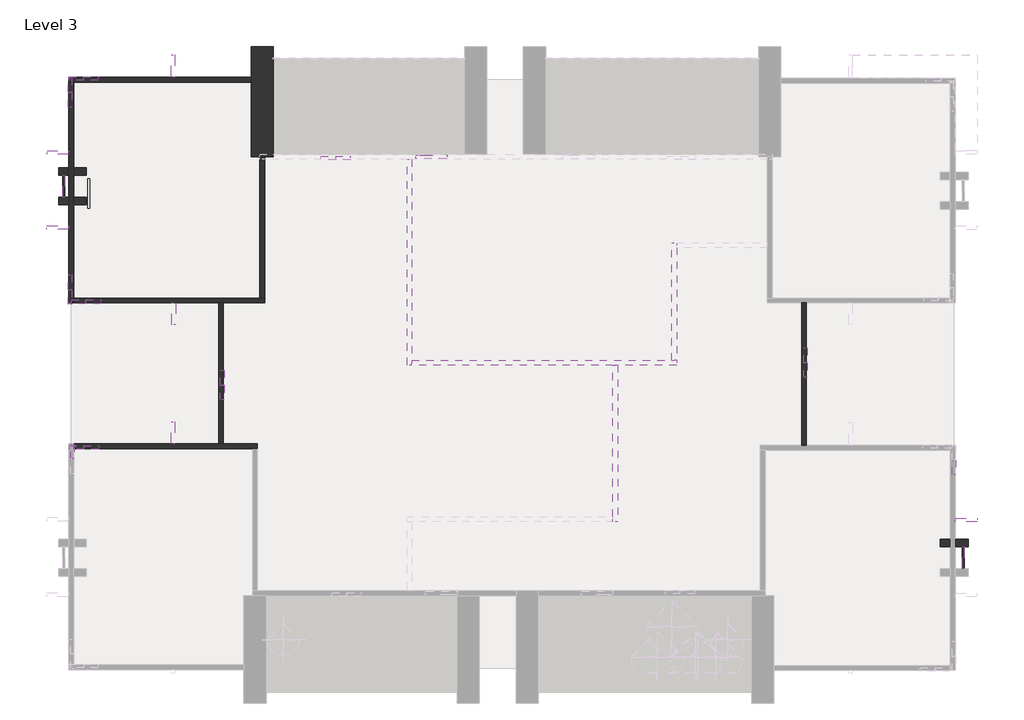
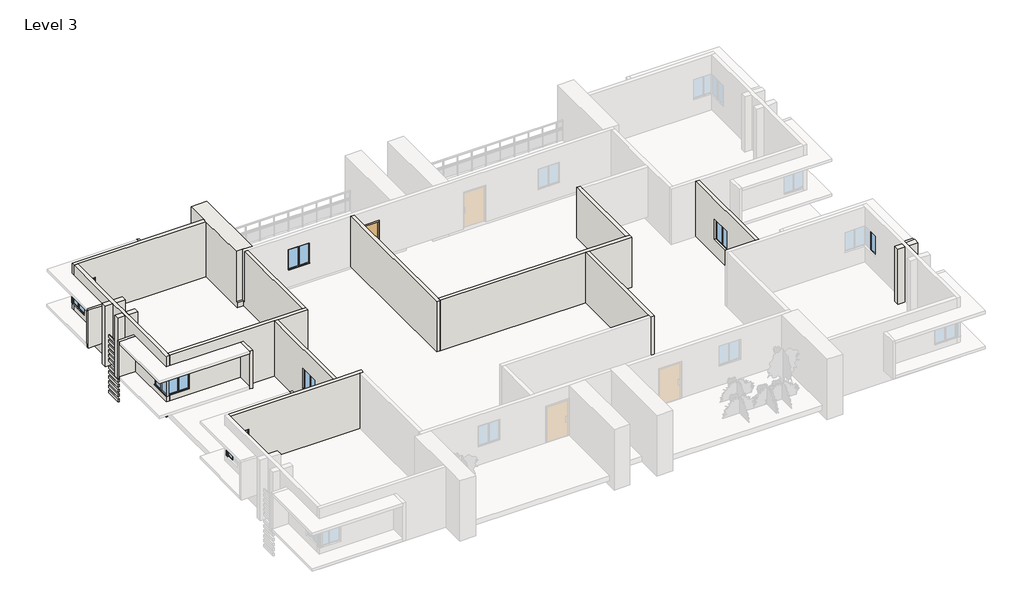
# One storey, part 2 of 4: 49 walls, 18 windows, 1 door.
"""IFC4 building model written with IfcOpenShell, lengths in millimetres."""

from ifc_helpers import new_model, si_unit, frame, origin, place, context, project, spatial, polyline, outline, extrude, faceted_brep, transform, mapped, element, save
from components import door_15d3c954, window_20ff4747

model = new_model("IFC4")

# Units and contexts
model_context = context("Model", 3, world=origin())
ifc_project = project(units=[si_unit("LENGTHUNIT", "METRE", prefix="MILLI")], contexts=[model_context])

# Site, building, storey
site = spatial("IfcSite", under=ifc_project)
building = spatial("IfcBuilding", under=site)
storey = spatial("IfcBuildingStorey", under=building, Name="Level 3", Elevation=6096.0)

# Door
placement = place(None, origin())
door_shape = door_15d3c954(model_context)
element("IfcDoor", 1, ObjectType="Door-Passage-Single-Flush-Dbl_Acting : 48\" x 96\"", at=placement, inside=storey, context=model_context, shape_type="MappedRepresentation", body=[
    mapped(door_shape, transform((153.0520665, 12804.5205944, 7315.2), x_axis=(1.0, 0.0, 0.0), y_axis=(0.0, 1.0, 0.0), z_axis=(0.0, 0.0, 1.0))),
])

# Walls
element("IfcWall", 2, ObjectType="Generic - 1'", at=placement, inside=storey, context=model_context, shape_type="SweptSolid", body=[
    extrude(outline(polyline([(-14151.7972154, 12048.8705944), (-14667.8479335, 12048.8705944), (-14667.8479335, 12353.6705944), (-14151.7972154, 12353.6705944), (-14151.7972154, 12048.8705944)])), frame((0.0, 0.0, 6705.6), z_axis=(0.0, 0.0, 1.0), x_axis=(1.0, 0.0, 0.0)), (0.0, 0.0, 1.0), 3657.6),
])
element("IfcWall", 3, ObjectType="Generic - 1'", at=placement, inside=storey, context=model_context, shape_type="SweptSolid", body=[
    extrude(outline(polyline([(-15302.1394029, 12353.6705944), (-14871.0479335, 12353.6705944), (-14871.0479335, 12048.8705944), (-15302.1394029, 12048.8705944), (-15302.1394029, 12353.6705944)])), frame((0.0, 0.0, 6705.6), z_axis=(0.0, 0.0, 1.0), x_axis=(1.0, 0.0, 0.0)), (0.0, 0.0, 1.0), 3657.6),
])
element("IfcWall", 4, ObjectType="Generic - 1'", at=placement, inside=storey, context=model_context, shape_type="SweptSolid", body=[
    extrude(outline(polyline([(-14151.7972154, 10829.6705944), (-14667.8479335, 10829.6705944), (-14667.8479335, 11134.4705944), (-14151.7972154, 11134.4705944), (-14151.7972154, 10829.6705944)])), frame((0.0, 0.0, 6705.6), z_axis=(0.0, 0.0, 1.0), x_axis=(1.0, 0.0, 0.0)), (0.0, 0.0, 1.0), 3657.6),
])
element("IfcWall", 5, ObjectType="Generic - 1'", at=placement, inside=storey, context=model_context, shape_type="SweptSolid", body=[
    extrude(outline(polyline([(-15302.1394029, 11134.4705944), (-14871.0479335, 11134.4705944), (-14871.0479335, 10829.6705944), (-15302.1394029, 10829.6705944), (-15302.1394029, 11134.4705944)])), frame((0.0, 0.0, 6705.6), z_axis=(0.0, 0.0, 1.0), x_axis=(1.0, 0.0, 0.0)), (0.0, 0.0, 1.0), 3657.6),
])
element("IfcWall", 6, ObjectType="Generic - 1'", at=placement, inside=storey, context=model_context, shape_type="SweptSolid", body=[
    extrude(outline(polyline([(22386.1027846, -3343.5294056), (21857.3520665, -3343.5294056), (21857.3520665, -3038.7294056), (22386.1027846, -3038.7294056), (22386.1027846, -3343.5294056)])), frame((0.0, 0.0, 6705.6), z_axis=(0.0, 0.0, 1.0), x_axis=(1.0, 0.0, 0.0)), (0.0, 0.0, 1.0), 3657.6),
])
element("IfcWall", 7, ObjectType="Generic - 1'", at=placement, inside=storey, context=model_context, shape_type="SweptSolid", body=[
    extrude(outline(polyline([(21235.7605971, -3038.7294056), (21654.1520665, -3038.7294056), (21654.1520665, -3343.5294056), (21235.7605971, -3343.5294056), (21235.7605971, -3038.7294056)])), frame((0.0, 0.0, 6705.6), z_axis=(0.0, 0.0, 1.0), x_axis=(1.0, 0.0, 0.0)), (0.0, 0.0, 1.0), 3657.6),
])
element("IfcWall", 8, ObjectType="Generic - 3'", at=placement, inside=storey, context=model_context, shape_type="Brep", body=[
    faceted_brep([(-6400.1479335, 12810.8705944, 6705.6), (-6400.1479335, 17382.8705944, 6705.6), (-6400.1479335, 17382.8705944, 10363.2), (-6400.1479335, 12912.4705944, 10363.2), (-6400.1479335, 12912.4705944, 7315.2), (-6400.1479335, 12810.8705944, 7315.2), (-7314.5479335, 12810.8705944, 6705.6), (-7314.5479335, 12810.8705944, 7315.2), (-7314.5479335, 12912.4705944, 7315.2), (-7314.5479335, 12912.4705944, 10363.2), (-7314.5479335, 15904.9548886, 10363.2), (-7314.5479335, 16108.1548886, 10363.2), (-7314.5479335, 17382.8705944, 10363.2), (-7314.5479335, 17382.8705944, 6705.6), (-7314.5479335, 16108.1548886, 6705.6), (-7314.5479335, 15904.9548886, 6705.6), (-6755.7479335, 12810.8705944, 6705.6), (-6958.9479335, 12810.8705944, 6705.6), (-6958.9479335, 12912.4705944, 10363.2), (-6755.7479335, 12810.8705944, 7315.2), (-6958.9479335, 12810.8705944, 7315.2), (-6958.9479335, 12912.4705944, 7315.2)], [[[0, 1, 2, 3, 4, 5]], [[6, 7, 8, 9, 10, 11, 12, 13, 14, 15]], [[1, 0, 16, 17, 6, 15, 14, 13]], [[2, 1, 13, 12]], [[3, 2, 12, 11, 10, 9, 18]], [[0, 5, 19, 20, 7, 6, 17, 16]], [[4, 21, 8, 7, 20, 19, 5]], [[4, 3, 18, 9, 8, 21]]]),
])
element("IfcWall", 9, ObjectType="Generic - 5\"", at=placement, inside=storey, context=model_context, shape_type="SweptSolid", body=[
    extrude(outline(polyline([(-15124.6936682, 11134.4705944), (-15124.6936682, 12048.8705944), (-15048.4936682, 12048.8705944), (-15048.4936682, 11134.4705944), (-15124.6936682, 11134.4705944)])), frame((0.0, 0.0, 5054.6), z_axis=(0.0, 0.0, 1.0), x_axis=(1.0, 0.0, 0.0)), (0.0, 0.0, 1.0), 152.8735856),
])
element("IfcWall", 10, ObjectType="Generic - 5\"", at=placement, inside=storey, context=model_context, shape_type="SweptSolid", body=[
    extrude(outline(polyline([(-15124.6936682, 11134.4705944), (-15124.6936682, 12048.8705944), (-15048.4936682, 12048.8705944), (-15048.4936682, 11134.4705944), (-15124.6936682, 11134.4705944)])), frame((0.0, 0.0, 5359.4), z_axis=(0.0, 0.0, 1.0), x_axis=(1.0, 0.0, 0.0)), (0.0, 0.0, 1.0), 152.8735856),
])
element("IfcWall", 11, ObjectType="Generic - 5\"", at=placement, inside=storey, context=model_context, shape_type="SweptSolid", body=[
    extrude(outline(polyline([(-15124.6936682, 11134.4705944), (-15124.6936682, 12048.8705944), (-15048.4936682, 12048.8705944), (-15048.4936682, 11134.4705944), (-15124.6936682, 11134.4705944)])), frame((0.0, 0.0, 5638.8), z_axis=(0.0, 0.0, 1.0), x_axis=(1.0, 0.0, 0.0)), (0.0, 0.0, 1.0), 152.8735856),
])
element("IfcWall", 12, ObjectType="Generic - 5\"", at=placement, inside=storey, context=model_context, shape_type="SweptSolid", body=[
    extrude(outline(polyline([(-15124.6936682, 11134.4705944), (-15124.6936682, 12048.8705944), (-15048.4936682, 12048.8705944), (-15048.4936682, 11134.4705944), (-15124.6936682, 11134.4705944)])), frame((0.0, 0.0, 5943.6), z_axis=(0.0, 0.0, 1.0), x_axis=(1.0, 0.0, 0.0)), (0.0, 0.0, 1.0), 152.8735856),
])
element("IfcWall", 13, ObjectType="Generic - 5\"", at=placement, inside=storey, context=model_context, shape_type="SweptSolid", body=[
    extrude(outline(polyline([(-15124.6936682, 11134.4705944), (-15124.6936682, 12048.8705944), (-15048.4936682, 12048.8705944), (-15048.4936682, 11134.4705944), (-15124.6936682, 11134.4705944)])), frame((0.0, 0.0, 6248.4), z_axis=(0.0, 0.0, 1.0), x_axis=(1.0, 0.0, 0.0)), (0.0, 0.0, 1.0), 152.8735856),
])
element("IfcWall", 14, ObjectType="Generic - 5\"", at=placement, inside=storey, context=model_context, shape_type="SweptSolid", body=[
    extrude(outline(polyline([(-15124.6936682, 11134.4705944), (-15124.6936682, 12048.8705944), (-15048.4936682, 12048.8705944), (-15048.4936682, 11134.4705944), (-15124.6936682, 11134.4705944)])), frame((0.0, 0.0, 6553.2), z_axis=(0.0, 0.0, 1.0), x_axis=(1.0, 0.0, 0.0)), (0.0, 0.0, 1.0), 152.8735856),
])
element("IfcWall", 15, ObjectType="Generic - 5\"", at=placement, inside=storey, context=model_context, shape_type="SweptSolid", body=[
    extrude(outline(polyline([(22145.9857703, -4257.9294056), (22145.9857703, -3343.5294056), (22222.1857703, -3343.5294056), (22222.1857703, -4257.9294056), (22145.9857703, -4257.9294056)])), frame((0.0, 0.0, 5054.6), z_axis=(0.0, 0.0, 1.0), x_axis=(1.0, 0.0, 0.0)), (0.0, 0.0, 1.0), 152.8735856),
])
element("IfcWall", 16, ObjectType="Generic - 5\"", at=placement, inside=storey, context=model_context, shape_type="SweptSolid", body=[
    extrude(outline(polyline([(22145.9857703, -4257.9294056), (22145.9857703, -3343.5294056), (22222.1857703, -3343.5294056), (22222.1857703, -4257.9294056), (22145.9857703, -4257.9294056)])), frame((0.0, 0.0, 5359.4), z_axis=(0.0, 0.0, 1.0), x_axis=(1.0, 0.0, 0.0)), (0.0, 0.0, 1.0), 152.8735856),
])
element("IfcWall", 17, ObjectType="Generic - 5\"", at=placement, inside=storey, context=model_context, shape_type="SweptSolid", body=[
    extrude(outline(polyline([(22145.9857703, -4257.9294056), (22145.9857703, -3343.5294056), (22222.1857703, -3343.5294056), (22222.1857703, -4257.9294056), (22145.9857703, -4257.9294056)])), frame((0.0, 0.0, 5638.8), z_axis=(0.0, 0.0, 1.0), x_axis=(1.0, 0.0, 0.0)), (0.0, 0.0, 1.0), 152.8735856),
])
element("IfcWall", 18, ObjectType="Generic - 5\"", at=placement, inside=storey, context=model_context, shape_type="SweptSolid", body=[
    extrude(outline(polyline([(22145.9857703, -4257.9294056), (22145.9857703, -3343.5294056), (22222.1857703, -3343.5294056), (22222.1857703, -4257.9294056), (22145.9857703, -4257.9294056)])), frame((0.0, 0.0, 5943.6), z_axis=(0.0, 0.0, 1.0), x_axis=(1.0, 0.0, 0.0)), (0.0, 0.0, 1.0), 152.8735856),
])
element("IfcWall", 19, ObjectType="Generic - 5\"", at=placement, inside=storey, context=model_context, shape_type="SweptSolid", body=[
    extrude(outline(polyline([(22145.9857703, -4257.9294056), (22145.9857703, -3343.5294056), (22222.1857703, -3343.5294056), (22222.1857703, -4257.9294056), (22145.9857703, -4257.9294056)])), frame((0.0, 0.0, 6248.4), z_axis=(0.0, 0.0, 1.0), x_axis=(1.0, 0.0, 0.0)), (0.0, 0.0, 1.0), 152.8735856),
])
element("IfcWall", 20, ObjectType="Generic - 5\"", at=placement, inside=storey, context=model_context, shape_type="SweptSolid", body=[
    extrude(outline(polyline([(22145.9857703, -4257.9294056), (22145.9857703, -3343.5294056), (22222.1857703, -3343.5294056), (22222.1857703, -4257.9294056), (22145.9857703, -4257.9294056)])), frame((0.0, 0.0, 6553.2), z_axis=(0.0, 0.0, 1.0), x_axis=(1.0, 0.0, 0.0)), (0.0, 0.0, 1.0), 152.8735856),
])
element("IfcWall", 21, ObjectType="Generic - 5\"", at=placement, inside=storey, context=model_context, shape_type="SweptSolid", body=[
    extrude(outline(polyline([(-15124.6936682, 11134.4705944), (-15124.6936682, 12048.8705944), (-15048.4936682, 12048.8705944), (-15048.4936682, 11134.4705944), (-15124.6936682, 11134.4705944)])), frame((0.0, 0.0, 6959.6), z_axis=(0.0, 0.0, 1.0), x_axis=(1.0, 0.0, 0.0)), (0.0, 0.0, 1.0), 152.8735856),
])
element("IfcWall", 22, ObjectType="Generic - 5\"", at=placement, inside=storey, context=model_context, shape_type="SweptSolid", body=[
    extrude(outline(polyline([(-14084.4224108, 10677.2705944), (-14084.4224108, 11896.4705944), (-14008.2224108, 11896.4705944), (-14008.2224108, 10677.2705944), (-14084.4224108, 10677.2705944)])), frame((0.0, 0.0, 6959.6), z_axis=(0.0, 0.0, 1.0), x_axis=(1.0, 0.0, 0.0)), (0.0, 0.0, 1.0), 178.1810075),
])
element("IfcWall", 23, ObjectType="Generic - 5\"", at=placement, inside=storey, context=model_context, shape_type="SweptSolid", body=[
    extrude(outline(polyline([(-15124.6936682, 11134.4705944), (-15124.6936682, 12048.8705944), (-15048.4936682, 12048.8705944), (-15048.4936682, 11134.4705944), (-15124.6936682, 11134.4705944)])), frame((0.0, 0.0, 7239.0), z_axis=(0.0, 0.0, 1.0), x_axis=(1.0, 0.0, 0.0)), (0.0, 0.0, 1.0), 152.8735856),
])
element("IfcWall", 24, ObjectType="Generic - 5\"", at=placement, inside=storey, context=model_context, shape_type="SweptSolid", body=[
    extrude(outline(polyline([(-15124.6936682, 11134.4705944), (-15124.6936682, 12048.8705944), (-15048.4936682, 12048.8705944), (-15048.4936682, 11134.4705944), (-15124.6936682, 11134.4705944)])), frame((0.0, 0.0, 7518.4), z_axis=(0.0, 0.0, 1.0), x_axis=(1.0, 0.0, 0.0)), (0.0, 0.0, 1.0), 152.8735856),
])
element("IfcWall", 25, ObjectType="Generic - 5\"", at=placement, inside=storey, context=model_context, shape_type="SweptSolid", body=[
    extrude(outline(polyline([(-15124.6936682, 11134.4705944), (-15124.6936682, 12048.8705944), (-15048.4936682, 12048.8705944), (-15048.4936682, 11134.4705944), (-15124.6936682, 11134.4705944)])), frame((0.0, 0.0, 7823.2), z_axis=(0.0, 0.0, 1.0), x_axis=(1.0, 0.0, 0.0)), (0.0, 0.0, 1.0), 152.8735856),
])
element("IfcWall", 26, ObjectType="Generic - 5\"", at=placement, inside=storey, context=model_context, shape_type="SweptSolid", body=[
    extrude(outline(polyline([(-15124.6936682, 11134.4705944), (-15124.6936682, 12048.8705944), (-15048.4936682, 12048.8705944), (-15048.4936682, 11134.4705944), (-15124.6936682, 11134.4705944)])), frame((0.0, 0.0, 8128.0), z_axis=(0.0, 0.0, 1.0), x_axis=(1.0, 0.0, 0.0)), (0.0, 0.0, 1.0), 152.8735856),
])
element("IfcWall", 27, ObjectType="Generic - 5\"", at=placement, inside=storey, context=model_context, shape_type="SweptSolid", body=[
    extrude(outline(polyline([(-15124.6936682, 11134.4705944), (-15124.6936682, 12048.8705944), (-15048.4936682, 12048.8705944), (-15048.4936682, 11134.4705944), (-15124.6936682, 11134.4705944)])), frame((0.0, 0.0, 8407.4), z_axis=(0.0, 0.0, 1.0), x_axis=(1.0, 0.0, 0.0)), (0.0, 0.0, 1.0), 152.8735856),
])
element("IfcWall", 28, ObjectType="Generic - 5\"", at=placement, inside=storey, context=model_context, shape_type="SweptSolid", body=[
    extrude(outline(polyline([(22145.9857703, -4257.9294056), (22145.9857703, -3343.5294056), (22222.1857703, -3343.5294056), (22222.1857703, -4257.9294056), (22145.9857703, -4257.9294056)])), frame((0.0, 0.0, 6959.6), z_axis=(0.0, 0.0, 1.0), x_axis=(1.0, 0.0, 0.0)), (0.0, 0.0, 1.0), 152.8735856),
])
element("IfcWall", 29, ObjectType="Generic - 5\"", at=placement, inside=storey, context=model_context, shape_type="SweptSolid", body=[
    extrude(outline(polyline([(22145.9857703, -4257.9294056), (22145.9857703, -3343.5294056), (22222.1857703, -3343.5294056), (22222.1857703, -4257.9294056), (22145.9857703, -4257.9294056)])), frame((0.0, 0.0, 7239.0), z_axis=(0.0, 0.0, 1.0), x_axis=(1.0, 0.0, 0.0)), (0.0, 0.0, 1.0), 152.8735856),
])
element("IfcWall", 30, ObjectType="Generic - 5\"", at=placement, inside=storey, context=model_context, shape_type="SweptSolid", body=[
    extrude(outline(polyline([(22145.9857703, -4257.9294056), (22145.9857703, -3343.5294056), (22222.1857703, -3343.5294056), (22222.1857703, -4257.9294056), (22145.9857703, -4257.9294056)])), frame((0.0, 0.0, 7518.4), z_axis=(0.0, 0.0, 1.0), x_axis=(1.0, 0.0, 0.0)), (0.0, 0.0, 1.0), 152.8735856),
])
element("IfcWall", 31, ObjectType="Generic - 5\"", at=placement, inside=storey, context=model_context, shape_type="SweptSolid", body=[
    extrude(outline(polyline([(22145.9857703, -4257.9294056), (22145.9857703, -3343.5294056), (22222.1857703, -3343.5294056), (22222.1857703, -4257.9294056), (22145.9857703, -4257.9294056)])), frame((0.0, 0.0, 7823.2), z_axis=(0.0, 0.0, 1.0), x_axis=(1.0, 0.0, 0.0)), (0.0, 0.0, 1.0), 152.8735856),
])
element("IfcWall", 32, ObjectType="Generic - 5\"", at=placement, inside=storey, context=model_context, shape_type="SweptSolid", body=[
    extrude(outline(polyline([(22145.9857703, -4257.9294056), (22145.9857703, -3343.5294056), (22222.1857703, -3343.5294056), (22222.1857703, -4257.9294056), (22145.9857703, -4257.9294056)])), frame((0.0, 0.0, 8128.0), z_axis=(0.0, 0.0, 1.0), x_axis=(1.0, 0.0, 0.0)), (0.0, 0.0, 1.0), 152.8735856),
])
element("IfcWall", 33, ObjectType="Generic - 5\"", at=placement, inside=storey, context=model_context, shape_type="SweptSolid", body=[
    extrude(outline(polyline([(22145.9857703, -4257.9294056), (22145.9857703, -3343.5294056), (22222.1857703, -3343.5294056), (22222.1857703, -4257.9294056), (22145.9857703, -4257.9294056)])), frame((0.0, 0.0, 8407.4), z_axis=(0.0, 0.0, 1.0), x_axis=(1.0, 0.0, 0.0)), (0.0, 0.0, 1.0), 152.8735856),
])
element("IfcWall", 34, ObjectType="Generic - 6\"", at=placement, inside=storey, context=model_context, shape_type="SweptSolid", body=[
    extrude(outline(polyline([(-10480.7034654, 17035.2548886), (-10480.7034654, 16120.8548886), (-10633.1034654, 16120.8548886), (-10633.1034654, 17035.2548886), (-10480.7034654, 17035.2548886)])), frame((0.0, 0.0, 7467.6), z_axis=(0.0, 0.0, 1.0), x_axis=(1.0, 0.0, 0.0)), (0.0, 0.0, 1.0), 2286.0),
])
element("IfcWall", 35, ObjectType="Generic - 6\"", at=placement, inside=storey, context=model_context, shape_type="SweptSolid", body=[
    extrude(outline(polyline([(-15775.8097154, 13072.8548886), (-14883.7479335, 13072.8548886), (-14883.7479335, 12920.4548886), (-15775.8097154, 12920.4548886), (-15775.8097154, 13072.8548886)])), frame((0.0, 0.0, 7467.6), z_axis=(0.0, 0.0, 1.0), x_axis=(1.0, 0.0, 0.0)), (0.0, 0.0, 1.0), 2286.0),
])
element("IfcWall", 36, ObjectType="Generic - 6\"", at=placement, inside=storey, context=model_context, shape_type="SweptSolid", body=[
    extrude(outline(polyline([(-10603.8479335, 5846.5548886), (-10603.8479335, 6760.9548886), (-10451.4479335, 6760.9548886), (-10451.4479335, 5846.5548886), (-10603.8479335, 5846.5548886)])), frame((0.0, 0.0, 7467.6), z_axis=(0.0, 0.0, 1.0), x_axis=(1.0, 0.0, 0.0)), (0.0, 0.0, 1.0), 2286.0),
])
element("IfcWall", 37, ObjectType="Generic - 6\"", at=placement, inside=storey, context=model_context, shape_type="SweptSolid", body=[
    extrude(outline(polyline([(-15798.1479335, 9961.3548886), (-14883.7479335, 9961.3548886), (-14883.7479335, 9808.9548886), (-15798.1479335, 9808.9548886), (-15798.1479335, 9961.3548886)])), frame((0.0, 0.0, 7467.6), z_axis=(0.0, 0.0, 1.0), x_axis=(1.0, 0.0, 0.0)), (0.0, 0.0, 1.0), 2286.0),
])
element("IfcWall", 38, ObjectType="Generic - 6\"", at=placement, inside=storey, context=model_context, shape_type="SweptSolid", body=[
    extrude(outline(polyline([(-10480.7034654, 1834.0395301), (-10480.7034654, 919.6395301), (-10633.1034654, 919.6395301), (-10633.1034654, 1834.0395301), (-10480.7034654, 1834.0395301)])), frame((0.0, 0.0, 7467.6), z_axis=(0.0, 0.0, 1.0), x_axis=(1.0, 0.0, 0.0)), (0.0, 0.0, 1.0), 2286.0),
])
element("IfcWall", 39, ObjectType="Generic - 6\"", at=placement, inside=storey, context=model_context, shape_type="SweptSolid", body=[
    extrude(outline(polyline([(22771.7520665, -2309.5899195), (21857.3520665, -2309.5899195), (21857.3520665, -2157.1899195), (22771.7520665, -2157.1899195), (22771.7520665, -2309.5899195)])), frame((0.0, 0.0, 7467.6), z_axis=(0.0, 0.0, 1.0), x_axis=(1.0, 0.0, 0.0)), (0.0, 0.0, 1.0), 2286.0),
])
element("IfcWall", 40, ObjectType="Generic - 8\"", at=placement, inside=storey, context=model_context, shape_type="Brep", body=[
    faceted_brep([(-862.9479335, 12709.2705944, 7315.2), (-862.9479335, 4174.8705944, 7315.2), (-862.9479335, 4174.8705944, 10363.2), (-862.9479335, 12709.2705944, 10363.2), (-659.7479335, 12709.2705944, 7315.2), (-659.7479335, 12709.2705944, 10363.2), (-659.7479335, 4378.0705944, 10363.2), (-659.7479335, 4174.8705944, 10363.2), (-659.7479335, 4174.8705944, 7315.2), (-659.7479335, 4378.0705944, 7315.2)], [[[0, 1, 2, 3]], [[4, 5, 6, 7, 8, 9]], [[1, 0, 4, 9, 8]], [[3, 2, 7, 6, 5]], [[0, 3, 5, 4]], [[2, 1, 8, 7]]]),
])
element("IfcWall", 41, ObjectType="Generic - 8\"", at=placement, inside=storey, context=model_context, shape_type="Brep", body=[
    faceted_brep([(-659.7479335, 4174.8705944, 7315.2), (7671.4520665, 4174.8705944, 7315.2), (7874.6520665, 4174.8705944, 7315.2), (10313.0520665, 4174.8705944, 7315.2), (10313.0520665, 4174.8705944, 10363.2), (7874.6520665, 4174.8705944, 10363.2), (7671.4520665, 4174.8705944, 10363.2), (-659.7479335, 4174.8705944, 10363.2), (-659.7479335, 4378.0705944, 7315.2), (-659.7479335, 4378.0705944, 10363.2), (10109.8520665, 4378.0705944, 10363.2), (10313.0520665, 4378.0705944, 10363.2), (10313.0520665, 4378.0705944, 7315.2), (10109.8520665, 4378.0705944, 7315.2)], [[[0, 1, 2, 3, 4, 5, 6, 7]], [[8, 9, 10, 11, 12, 13]], [[3, 2, 1, 0, 8, 13, 12]], [[7, 6, 5, 4, 11, 10, 9]], [[0, 7, 9, 8]], [[4, 3, 12, 11]]]),
])
element("IfcWall", 42, ObjectType="Generic - 8\"", at=placement, inside=storey, context=model_context, shape_type="Brep", body=[
    faceted_brep([(10313.0520665, 4378.0705944, 7315.2), (10313.0520665, 9051.6705944, 7315.2), (10313.0520665, 9254.8705944, 7315.2), (10313.0520665, 9254.8705944, 10363.2), (10313.0520665, 9051.6705944, 10363.2), (10313.0520665, 4378.0705944, 10363.2), (10109.8520665, 4378.0705944, 7315.2), (10109.8520665, 4378.0705944, 10363.2), (10109.8520665, 9254.8705944, 10363.2), (10109.8520665, 9254.8705944, 7315.2)], [[[0, 1, 2, 3, 4, 5]], [[6, 7, 8, 9]], [[2, 1, 0, 6, 9]], [[5, 4, 3, 8, 7]], [[0, 5, 7, 6]], [[3, 2, 9, 8]]]),
])
element("IfcWall", 43, ObjectType="Generic - 8\"", at=placement, inside=storey, context=model_context, shape_type="Brep", body=[
    faceted_brep([(7671.4520665, 4174.8705944, 7315.2), (7671.4520665, -2102.9604699, 7315.2), (7671.4520665, -2306.1604699, 7315.2), (7671.4520665, -2306.1604699, 10363.2), (7671.4520665, -2102.9604699, 10363.2), (7671.4520665, 4174.8705944, 10363.2), (7874.6520665, 4174.8705944, 7315.2), (7874.6520665, 4174.8705944, 10363.2), (7874.6520665, -2306.1604699, 10363.2), (7874.6520665, -2306.1604699, 7315.2)], [[[0, 1, 2, 3, 4, 5]], [[6, 7, 8, 9]], [[2, 1, 0, 6, 9]], [[5, 4, 3, 8, 7]], [[0, 5, 7, 6]], [[3, 2, 9, 8]]]),
])
element("IfcWall", 44, ObjectType="Generic - 8\" gray", at=placement, inside=storey, context=model_context, shape_type="Brep", body=[
    faceted_brep([(-14871.0479335, 15904.9548886, 6705.6), (-14667.8479335, 15904.9548886, 6705.6), (-7314.5479335, 15904.9548886, 6705.6), (-7314.5479335, 15904.9548886, 10363.2), (-14667.8479335, 15904.9548886, 10363.2), (-14871.0479335, 15904.9548886, 10363.2), (-14871.0479335, 15904.9548886, 9197.0804451), (-14667.8479335, 15904.9548886, 9197.0804451), (-13661.292575, 15904.9548886, 9197.0804451), (-13661.292575, 15904.9548886, 7977.8804451), (-14667.8479335, 15904.9548886, 7977.8804451), (-14871.0479335, 15904.9548886, 7977.8804451), (-7314.5479335, 16108.1548886, 6705.6), (-14871.0479335, 16108.1548886, 6705.6), (-14871.0479335, 16108.1548886, 7977.8804451), (-13661.292575, 16108.1548886, 7977.8804451), (-13661.292575, 16108.1548886, 9197.0804451), (-14871.0479335, 16108.1548886, 9197.0804451), (-14871.0479335, 16108.1548886, 10363.2), (-7314.5479335, 16108.1548886, 10363.2)], [[[0, 1, 2, 3, 4, 5, 6, 7, 8, 9, 10, 11]], [[12, 13, 14, 15, 16, 17, 18, 19]], [[2, 1, 0, 13, 12]], [[5, 4, 3, 19, 18]], [[5, 18, 17, 6]], [[13, 0, 11, 14]], [[3, 2, 12, 19]], [[9, 15, 14, 11, 10]], [[6, 17, 16, 8, 7]], [[8, 16, 15, 9]]]),
])
element("IfcWall", 45, ObjectType="Generic - 8\" gray", at=placement, inside=storey, context=model_context, shape_type="Brep", body=[
    faceted_brep([(-14667.8479335, 6760.9548886, 6705.6), (-14667.8479335, 6964.1548886, 6705.6), (-14667.8479335, 10829.6705944, 6705.6), (-14667.8479335, 11134.4705944, 6705.6), (-14667.8479335, 12048.8705944, 6705.6), (-14667.8479335, 12353.6705944, 6705.6), (-14667.8479335, 15904.9548886, 6705.6), (-14667.8479335, 15904.9548886, 7977.8804451), (-14667.8479335, 14871.0236266, 7977.8804451), (-14667.8479335, 14871.0236266, 9197.0804451), (-14667.8479335, 15904.9548886, 9197.0804451), (-14667.8479335, 15904.9548886, 10363.2), (-14667.8479335, 12353.6705944, 10363.2), (-14667.8479335, 12048.8705944, 10363.2), (-14667.8479335, 11134.4705944, 10363.2), (-14667.8479335, 10829.6705944, 10363.2), (-14667.8479335, 6964.1548886, 10363.2), (-14667.8479335, 6760.9548886, 10363.2), (-14667.8479335, 6760.9548886, 9197.0804451), (-14667.8479335, 6964.1548886, 9197.0804451), (-14667.8479335, 7918.4820466, 9197.0804451), (-14667.8479335, 7918.4820466, 7977.8804451), (-14667.8479335, 6964.1548886, 7977.8804451), (-14667.8479335, 6760.9548886, 7977.8804451), (-14871.0479335, 15904.9548886, 6705.6), (-14871.0479335, 12353.6705944, 6705.6), (-14871.0479335, 12048.8705944, 6705.6), (-14871.0479335, 11134.4705944, 6705.6), (-14871.0479335, 10829.6705944, 6705.6), (-14871.0479335, 6760.9548886, 6705.6), (-14871.0479335, 6760.9548886, 7977.8804451), (-14871.0479335, 7918.4820466, 7977.8804451), (-14871.0479335, 7918.4820466, 9197.0804451), (-14871.0479335, 6760.9548886, 9197.0804451), (-14871.0479335, 6760.9548886, 10363.2), (-14871.0479335, 10829.6705944, 10363.2), (-14871.0479335, 11134.4705944, 10363.2), (-14871.0479335, 12048.8705944, 10363.2), (-14871.0479335, 12353.6705944, 10363.2), (-14871.0479335, 15904.9548886, 10363.2), (-14871.0479335, 15904.9548886, 9197.0804451), (-14871.0479335, 14871.0236266, 9197.0804451), (-14871.0479335, 14871.0236266, 7977.8804451), (-14871.0479335, 15904.9548886, 7977.8804451)], [[[0, 1, 2, 3, 4, 5, 6, 7, 8, 9, 10, 11, 12, 13, 14, 15, 16, 17, 18, 19, 20, 21, 22, 23]], [[24, 25, 26, 27, 28, 29, 30, 31, 32, 33, 34, 35, 36, 37, 38, 39, 40, 41, 42, 43]], [[6, 5, 4, 3, 2, 1, 0, 29, 28, 27, 26, 25, 24]], [[17, 16, 15, 14, 13, 12, 11, 39, 38, 37, 36, 35, 34]], [[17, 34, 33, 18]], [[29, 0, 23, 30]], [[6, 24, 43, 7]], [[39, 11, 10, 40]], [[30, 23, 22, 21, 31]], [[18, 33, 32, 20, 19]], [[20, 32, 31, 21]], [[7, 43, 42, 8]], [[9, 8, 42, 41]], [[9, 41, 40, 10]]]),
])
element("IfcWall", 46, ObjectType="Generic - 8\" gray", at=placement, inside=storey, context=model_context, shape_type="Brep", body=[
    faceted_brep([(-6755.7479335, 6964.1548886, 6705.6), (-6958.9479335, 6964.1548886, 6705.6), (-14667.8479335, 6964.1548886, 6705.6), (-14667.8479335, 6964.1548886, 7977.8804451), (-13556.3228261, 6964.1548886, 7977.8804451), (-13556.3228261, 6964.1548886, 9197.0804451), (-14667.8479335, 6964.1548886, 9197.0804451), (-14667.8479335, 6964.1548886, 10363.2), (-6958.9479335, 6964.1548886, 10363.2), (-6755.7479335, 6964.1548886, 10363.2), (-14667.8479335, 6760.9548886, 6705.6), (-8673.4479335, 6760.9548886, 6705.6), (-8470.2479335, 6760.9548886, 6705.6), (-6755.7479335, 6760.9548886, 6705.6), (-6755.7479335, 6760.9548886, 10363.2), (-8470.2479335, 6760.9548886, 10363.2), (-8673.4479335, 6760.9548886, 10363.2), (-14667.8479335, 6760.9548886, 10363.2), (-14667.8479335, 6760.9548886, 9197.0804451), (-13556.3228261, 6760.9548886, 9197.0804451), (-13556.3228261, 6760.9548886, 7977.8804451), (-14667.8479335, 6760.9548886, 7977.8804451)], [[[0, 1, 2, 3, 4, 5, 6, 7, 8, 9]], [[10, 11, 12, 13, 14, 15, 16, 17, 18, 19, 20, 21]], [[2, 1, 0, 13, 12, 11, 10]], [[9, 8, 7, 17, 16, 15, 14]], [[2, 10, 21, 3]], [[17, 7, 6, 18]], [[0, 9, 14, 13]], [[3, 21, 20, 4]], [[5, 4, 20, 19]], [[5, 19, 18, 6]]]),
])
element("IfcWall", 47, ObjectType="Generic - 8\" gray", at=placement, inside=storey, context=model_context, shape_type="Brep", body=[
    faceted_brep([(-7060.5479335, 919.6395301, 6705.6), (-8470.2479335, 919.6395301, 6705.6), (-8673.4479335, 919.6395301, 6705.6), (-14680.5479335, 919.6395301, 6705.6), (-14680.5479335, 919.6395301, 7977.8804451), (-13641.9760869, 919.6395301, 7977.8804451), (-13641.9760869, 919.6395301, 9197.0804451), (-14680.5479335, 919.6395301, 9197.0804451), (-14680.5479335, 919.6395301, 10363.2), (-8673.4479335, 919.6395301, 10363.2), (-8470.2479335, 919.6395301, 10363.2), (-7060.5479335, 919.6395301, 10363.2), (-14680.5479335, 716.4395301, 6705.6), (-7263.7479335, 716.4395301, 6705.6), (-7060.5479335, 716.4395301, 6705.6), (-7060.5479335, 716.4395301, 10363.2), (-7263.7479335, 716.4395301, 10363.2), (-14680.5479335, 716.4395301, 10363.2), (-14680.5479335, 716.4395301, 9197.0804451), (-13641.9760869, 716.4395301, 9197.0804451), (-13641.9760869, 716.4395301, 7977.8804451), (-14680.5479335, 716.4395301, 7977.8804451), (-14680.5479335, 908.9135189, 7977.8804451), (-14680.5479335, 908.9135189, 9197.0804451)], [[[0, 1, 2, 3, 4, 5, 6, 7, 8, 9, 10, 11]], [[12, 13, 14, 15, 16, 17, 18, 19, 20, 21]], [[3, 2, 1, 0, 14, 13, 12]], [[11, 10, 9, 8, 17, 16, 15]], [[3, 12, 21, 22, 4]], [[17, 8, 7, 23, 18]], [[0, 11, 15, 14]], [[4, 22, 21, 20, 5]], [[6, 5, 20, 19]], [[6, 19, 18, 23, 7]]]),
])
element("IfcWall", 48, ObjectType="Generic - 8\" gray", at=placement, inside=storey, context=model_context, shape_type="SweptSolid", body=[
    extrude(outline(polyline([(6760.9548886, 6705.6), (919.6395301, 6705.6), (919.6395301, 10363.2), (6760.9548886, 10363.2), (6760.9548886, 6705.6)]), holes=[polyline([(2742.9076732, 7977.8804451), (3962.1076732, 7977.8804451), (3962.1076732, 9197.0804451), (2742.9076732, 9197.0804451), (2742.9076732, 7977.8804451)])]), frame((-8673.4479335, 0.0, 0.0), z_axis=(1.0, 0.0, 0.0), x_axis=(0.0, 1.0, 0.0)), (0.0, 0.0, 1.0), 203.2),
])
element("IfcWall", 49, ObjectType="Generic - 8\" gray", at=placement, inside=storey, context=model_context, shape_type="SweptSolid", body=[
    extrude(outline(polyline([(6760.9548886, 6705.6), (868.1548886, 6705.6), (868.1548886, 10363.2), (6760.9548886, 10363.2), (6760.9548886, 6705.6)]), holes=[polyline([(3676.3636585, 7977.8804451), (4895.5636585, 7977.8804451), (4895.5636585, 9197.0804451), (3676.3636585, 9197.0804451), (3676.3636585, 7977.8804451)])]), frame((15481.9520665, 0.0, 0.0), z_axis=(1.0, 0.0, 0.0), x_axis=(0.0, 1.0, 0.0)), (0.0, 0.0, 1.0), 203.2),
])
element("IfcWall", 50, ObjectType="Generic - 8\" gray", at=placement, inside=storey, context=model_context, shape_type="SweptSolid", body=[
    extrude(outline(polyline([(6964.1548886, 6705.6), (6964.1548886, 10363.2), (12709.2705944, 10363.2), (12709.2705944, 7315.2), (12810.8705944, 7315.2), (12810.8705944, 6705.6), (6964.1548886, 6705.6)])), frame((-6958.9479335, 0.0, 0.0), z_axis=(1.0, 0.0, 0.0), x_axis=(0.0, 1.0, 0.0)), (0.0, 0.0, 1.0), 203.2),
])

# Windows
window_shape = window_20ff4747(model_context)
element("IfcWindow", 51, ObjectType="Instance - Fixed : 24\" x 48\"", at=placement, inside=storey, context=model_context, shape_type="MappedRepresentation", body=[
    mapped(window_shape, transform((21755.7520665, -93.135515, 7063.4804451), x_axis=(0.0, -1.0, 0.0), y_axis=(1.0, 0.0, 0.0), z_axis=(0.0, 0.0, 1.0))),
])
element("IfcWindow", 52, ObjectType="Instance - Fixed : 24\" x 48\"", at=placement, inside=storey, context=model_context, shape_type="MappedRepresentation", body=[
    mapped(window_shape, transform((-14782.1479335, 566.0135189, 7063.4804451), x_axis=(0.0, -1.0, 0.0), y_axis=(1.0, 0.0, 0.0), z_axis=(0.0, 0.0, 1.0))),
])
element("IfcWindow", 53, ObjectType="Instance - Fixed : 24\" x 48\"", at=placement, inside=storey, context=model_context, shape_type="MappedRepresentation", body=[
    mapped(window_shape, transform((-14594.4760869, 818.0395301, 7063.4804451), x_axis=(-1.0, 0.0, 0.0), y_axis=(0.0, -1.0, 0.0), z_axis=(0.0, 0.0, 1.0))),
])
element("IfcWindow", 54, ObjectType="Instance - Fixed : 24\" x 48\"", at=placement, inside=storey, context=model_context, shape_type="MappedRepresentation", body=[
    mapped(window_shape, transform((-13984.8760869, 818.0395301, 7063.4804451), x_axis=(-1.0, 0.0, 0.0), y_axis=(0.0, -1.0, 0.0), z_axis=(0.0, 0.0, 1.0))),
])
element("IfcWindow", 55, ObjectType="Instance - Fixed : 24\" x 48\"", at=placement, inside=storey, context=model_context, shape_type="MappedRepresentation", body=[
    mapped(window_shape, transform((-14508.8228261, 6862.5548886, 7063.4804451), x_axis=(-1.0, 0.0, 0.0), y_axis=(0.0, -1.0, 0.0), z_axis=(0.0, 0.0, 1.0))),
])
element("IfcWindow", 56, ObjectType="Instance - Fixed : 24\" x 48\"", at=placement, inside=storey, context=model_context, shape_type="MappedRepresentation", body=[
    mapped(window_shape, transform((-13899.2228261, 6862.5548886, 7063.4804451), x_axis=(-1.0, 0.0, 0.0), y_axis=(0.0, -1.0, 0.0), z_axis=(0.0, 0.0, 1.0))),
])
element("IfcWindow", 57, ObjectType="Instance - Fixed : 24\" x 48\"", at=placement, inside=storey, context=model_context, shape_type="MappedRepresentation", body=[
    mapped(window_shape, transform((-14769.4479335, 7651.7820466, 7063.4804451), x_axis=(0.0, 1.0, 0.0), y_axis=(-1.0, 0.0, 0.0), z_axis=(0.0, 0.0, 1.0))),
])
element("IfcWindow", 58, ObjectType="Instance - Fixed : 24\" x 48\"", at=placement, inside=storey, context=model_context, shape_type="MappedRepresentation", body=[
    mapped(window_shape, transform((-14769.4479335, 7042.1820466, 7063.4804451), x_axis=(0.0, 1.0, 0.0), y_axis=(-1.0, 0.0, 0.0), z_axis=(0.0, 0.0, 1.0))),
])
element("IfcWindow", 59, ObjectType="Instance - Fixed : 24\" x 48\"", at=placement, inside=storey, context=model_context, shape_type="MappedRepresentation", body=[
    mapped(window_shape, transform((-14769.4479335, 15823.5236266, 7063.4804451), x_axis=(0.0, 1.0, 0.0), y_axis=(-1.0, 0.0, 0.0), z_axis=(0.0, 0.0, 1.0))),
])
element("IfcWindow", 60, ObjectType="Instance - Fixed : 24\" x 48\"", at=placement, inside=storey, context=model_context, shape_type="MappedRepresentation", body=[
    mapped(window_shape, transform((-14769.4479335, 15213.9236266, 7063.4804451), x_axis=(0.0, 1.0, 0.0), y_axis=(-1.0, 0.0, 0.0), z_axis=(0.0, 0.0, 1.0))),
])
element("IfcWindow", 61, ObjectType="Instance - Fixed : 24\" x 48\"", at=placement, inside=storey, context=model_context, shape_type="MappedRepresentation", body=[
    mapped(window_shape, transform((-13927.992575, 16006.5548886, 7063.4804451), x_axis=(1.0, 0.0, 0.0), y_axis=(0.0, 1.0, 0.0), z_axis=(0.0, 0.0, 1.0))),
])
element("IfcWindow", 62, ObjectType="Instance - Fixed : 24\" x 48\"", at=placement, inside=storey, context=model_context, shape_type="MappedRepresentation", body=[
    mapped(window_shape, transform((-14537.592575, 16006.5548886, 7063.4804451), x_axis=(1.0, 0.0, 0.0), y_axis=(0.0, 1.0, 0.0), z_axis=(0.0, 0.0, 1.0))),
])
element("IfcWindow", 63, ObjectType="Instance - Fixed : 24\" x 48\"", at=placement, inside=storey, context=model_context, shape_type="MappedRepresentation", body=[
    mapped(window_shape, transform((-4165.821881, 12810.8705944, 7446.2298362), x_axis=(-1.0, 0.0, 0.0), y_axis=(0.0, -1.0, 0.0), z_axis=(0.0, 0.0, 1.0))),
])
element("IfcWindow", 64, ObjectType="Instance - Fixed : 24\" x 48\"", at=placement, inside=storey, context=model_context, shape_type="MappedRepresentation", body=[
    mapped(window_shape, transform((-3556.221881, 12810.8705944, 7446.2298362), x_axis=(-1.0, 0.0, 0.0), y_axis=(0.0, -1.0, 0.0), z_axis=(0.0, 0.0, 1.0))),
])
element("IfcWindow", 65, ObjectType="Instance - Fixed : 24\" x 48\"", at=placement, inside=storey, context=model_context, shape_type="MappedRepresentation", body=[
    mapped(window_shape, transform((-8571.8479335, 3009.6076732, 7063.4804451), x_axis=(0.0, -1.0, 0.0), y_axis=(1.0, 0.0, 0.0), z_axis=(0.0, 0.0, 1.0))),
])
element("IfcWindow", 66, ObjectType="Instance - Fixed : 24\" x 48\"", at=placement, inside=storey, context=model_context, shape_type="MappedRepresentation", body=[
    mapped(window_shape, transform((-8571.8479335, 3619.2076732, 7063.4804451), x_axis=(0.0, -1.0, 0.0), y_axis=(1.0, 0.0, 0.0), z_axis=(0.0, 0.0, 1.0))),
])
element("IfcWindow", 67, ObjectType="Instance - Fixed : 24\" x 48\"", at=placement, inside=storey, context=model_context, shape_type="MappedRepresentation", body=[
    mapped(window_shape, transform((15583.5520665, 3943.0636585, 7063.4804451), x_axis=(0.0, -1.0, 0.0), y_axis=(1.0, 0.0, 0.0), z_axis=(0.0, 0.0, 1.0))),
])
element("IfcWindow", 68, ObjectType="Instance - Fixed : 24\" x 48\"", at=placement, inside=storey, context=model_context, shape_type="MappedRepresentation", body=[
    mapped(window_shape, transform((15583.5520665, 4552.6636585, 7063.4804451), x_axis=(0.0, -1.0, 0.0), y_axis=(1.0, 0.0, 0.0), z_axis=(0.0, 0.0, 1.0))),
])

save(model, "model.ifc")

# Revit data of these elements
# Type "Door-Passage-Single-Flush-Dbl_Acting : 48\" x 96\""
#   Type Mark = "12"
#   Assembly Code = "B2030200"
#   Analytic Construction = "Wooden"
#   Thickness = 0' - 1 3/4"
#   Thermal Resistance (R) = 2.5876 (h·ft²·°F)/BTU
#   Swing Angle [instance default] = 45.00°
#   Strike Height = 3' - 4"
#   Rough Width [instance default] = 4' - 4"
#   Rough Height [instance default] = 7' - 4"
#   MF Opening Height [instance default] = 0' - 4"
#   MF Opening Width [instance default] = 0' - 4"
#   Inset Calculate [instance default] = 0' - 4"
#   Masonry Inset [instance default] = 0' - 1"
#   Height = 7' - 0"
#   Width = 4' - 0"
#   Heat Transfer Coefficient (U) = 0.3865 BTU/(h·ft²·°F)
#   Masonry Frame Depth = 0' - 5 3/4"
#   Masonry Frame [instance default] = yes
#   Function = 1
#   Dry Wall Frame [instance default] = no
#   Panel Material = Wood - Birch
#   Frame Material = Metal - Paint Finish - Grey
#   Door Handle Material = Aluminum
#   Visual Light Transmittance = 0
#   Solar Heat Gain Coefficient = 0
#   Wall Closure = (empty or 0)
# Type "Generic - 1'"
#   Assembly Code = "B2010"
#   Layers, outside or top first: 1' - 0" "Metal - Painted - Grey" (function 1)
# Type "Generic - 3'"
#   Assembly Code = "B2010"
#   Layers, outside or top first: 3' - 0" "Metal - Painted - Grey" (function 1)
# Type "Generic - 5\""
#   Assembly Code = "B2010"
#   Layers, outside or top first: 0' - 3" "Oak Flooring" (function 1)
# Type "Generic - 6\""
#   Assembly Code = "B2010"
#   Layers, outside or top first: 0' - 6" "Metal - Painted - Grey" (function 1)
# Type "Generic - 8\""
#   Assembly Code = "B2010"
#   Layers, outside or top first: 0' - 8" no material (function 1)
# Type "Generic - 8\" gray"
#   Assembly Code = "B2010"
#   Layers, outside or top first: 0' - 8" "Parking Stripe" (function 1)
# Type "Instance - Fixed : 24\" x 48\""
#   Type Mark = "11"
#   Construction Type Id = "GSP4R"
#   Assembly Code = "B2020100"
#   Analytic Construction = "1/8 in Pilkington single glazing"
#   Visual Light Transmittance = 0.9
#   Thermal Resistance (R) = 0.8466 (h·ft²·°F)/BTU
#   Solar Heat Gain Coefficient = 0.86
#   Heat Transfer Coefficient (U) = 1.1812 BTU/(h·ft²·°F)
#   Height [instance default] = 4' - 0"
#   Default Sill Height = 3' - 0"
#   Width [instance default] = 2' - 0"
#   Window Inset = 0' - 2"
#   Define Thermal Properties by = 1
#   Glass Pane Material = Glass
#   Sash Material = Iron, Ductile
#   Wall Closure = (empty or 0)
# Element 1 (IfcDoor, "Door-Passage-Single-Flush-Dbl_Acting : 48\" x 96\"")
#   Swing Angle = 45.00°
#   Rough Width = 4' - 4"
#   Rough Height = 7' - 4"
#   Masonry Inset = 0' - 1"
#   MF Opening Width = 0' - 4"
#   MF Opening Height = 0' - 4"
#   Inset Calculate = 0' - 4"
#   Masonry Frame = yes
#   Dry Wall Frame = no
#   Phase Created = New Construction
#   Materials on its faces: "Aluminum", "Metal - Paint Finish - Grey", "Wood - Birch"
# Elements 2, 3, 4, 5, 6, 7 (IfcWall, "Generic - 1'")
#   built-in parameter 1001111 = 2' - 0"
#   Top Offset = 0' - 0"
#   Base Offset = 2' - 0"
#   Unconnected Height = 12' - 0"
#   wall height = 12' - 0"
#   Phase Created = New Construction
#   Base Constraint = Level 3
#   Materials on its faces: "Metal - Painted - Grey"
# Element 8 (IfcWall, "Generic - 3'")
#   built-in parameter 1001111 = 2' - 0"
#   Top Offset = 0' - 0"
#   Base Offset = 2' - 0"
#   Unconnected Height = 12' - 0"
#   wall height = 12' - 0"
#   Phase Created = New Construction
#   Base Constraint = Level 3
#   Materials on its faces: "Metal - Painted - Grey", "EIFS, Exterior Insulation"
# Elements 9, 15 (IfcWall, "Generic - 5\"")
#   built-in parameter 1001111 = -3' - 5"
#   Top Offset = -12' - 10.98135"
#   Base Offset = -3' - 5"
#   wall height = 0' - 6.01865"
#   Phase Created = New Construction
#   Base Constraint = Level 3
#   Top Constraint = Level 4
#   Materials on its faces: "Oak Flooring"
# Elements 10, 16 (IfcWall, "Generic - 5\"")
#   built-in parameter 1001111 = -2' - 5"
#   Top Offset = -11' - 10.98135"
#   Base Offset = -2' - 5"
#   wall height = 0' - 6.01865"
#   Phase Created = New Construction
#   Base Constraint = Level 3
#   Top Constraint = Level 4
#   Materials on its faces: "Oak Flooring"
# Elements 11, 17 (IfcWall, "Generic - 5\"")
#   built-in parameter 1001111 = -1' - 6"
#   Top Offset = -10' - 11.98135"
#   Base Offset = -1' - 6"
#   wall height = 0' - 6.01865"
#   Phase Created = New Construction
#   Base Constraint = Level 3
#   Top Constraint = Level 4
#   Materials on its faces: "Oak Flooring"
# Elements 12, 18 (IfcWall, "Generic - 5\"")
#   built-in parameter 1001111 = -0' - 6"
#   Top Offset = -9' - 11.98135"
#   Base Offset = -0' - 6"
#   wall height = 0' - 6.01865"
#   Phase Created = New Construction
#   Base Constraint = Level 3
#   Top Constraint = Level 4
#   Materials on its faces: "Oak Flooring"
# Elements 13, 19 (IfcWall, "Generic - 5\"")
#   built-in parameter 1001111 = 0' - 6"
#   Top Offset = -8' - 11.98135"
#   Base Offset = 0' - 6"
#   wall height = 0' - 6.01865"
#   Phase Created = New Construction
#   Base Constraint = Level 3
#   Top Constraint = Level 4
#   Materials on its faces: "Oak Flooring"
# Elements 14, 20 (IfcWall, "Generic - 5\"")
#   built-in parameter 1001111 = 1' - 6"
#   Top Offset = -7' - 11.98135"
#   Base Offset = 1' - 6"
#   wall height = 0' - 6.01865"
#   Phase Created = New Construction
#   Base Constraint = Level 3
#   Top Constraint = Level 4
#   Materials on its faces: "Oak Flooring"
# Elements 21, 28 (IfcWall, "Generic - 5\"")
#   built-in parameter 1001111 = 2' - 10"
#   Top Offset = -6' - 7.98135"
#   Base Offset = 2' - 10"
#   wall height = 0' - 6.01865"
#   Phase Created = New Construction
#   Base Constraint = Level 3
#   Top Constraint = Level 4
#   Materials on its faces: "Oak Flooring"
# Element 22 (IfcWall, "Generic - 5\"")
#   built-in parameter 1001111 = 2' - 10"
#   Top Offset = -6' - 6.985"
#   Base Offset = 2' - 10"
#   wall height = 0' - 7.015"
#   Phase Created = New Construction
#   Base Constraint = Level 3
#   Top Constraint = Level 4
#   Materials on its faces: "Oak Flooring"
# Elements 23, 29 (IfcWall, "Generic - 5\"")
#   built-in parameter 1001111 = 3' - 9"
#   Top Offset = -5' - 8.98135"
#   Base Offset = 3' - 9"
#   wall height = 0' - 6.01865"
#   Phase Created = New Construction
#   Base Constraint = Level 3
#   Top Constraint = Level 4
#   Materials on its faces: "Oak Flooring"
# Elements 24, 30 (IfcWall, "Generic - 5\"")
#   built-in parameter 1001111 = 4' - 8"
#   Top Offset = -4' - 9.98135"
#   Base Offset = 4' - 8"
#   wall height = 0' - 6.01865"
#   Phase Created = New Construction
#   Base Constraint = Level 3
#   Top Constraint = Level 4
#   Materials on its faces: "Oak Flooring"
# Elements 25, 31 (IfcWall, "Generic - 5\"")
#   built-in parameter 1001111 = 5' - 8"
#   Top Offset = -3' - 9.98135"
#   Base Offset = 5' - 8"
#   wall height = 0' - 6.01865"
#   Phase Created = New Construction
#   Base Constraint = Level 3
#   Top Constraint = Level 4
#   Materials on its faces: "Oak Flooring"
# Elements 26, 32 (IfcWall, "Generic - 5\"")
#   built-in parameter 1001111 = 6' - 8"
#   Top Offset = -2' - 9.98135"
#   Base Offset = 6' - 8"
#   wall height = 0' - 6.01865"
#   Phase Created = New Construction
#   Base Constraint = Level 3
#   Top Constraint = Level 4
#   Materials on its faces: "Oak Flooring"
# Elements 27, 33 (IfcWall, "Generic - 5\"")
#   built-in parameter 1001111 = 7' - 7"
#   Top Offset = -1' - 10.98135"
#   Base Offset = 7' - 7"
#   wall height = 0' - 6.01865"
#   Phase Created = New Construction
#   Base Constraint = Level 3
#   Top Constraint = Level 4
#   Materials on its faces: "Oak Flooring"
# Elements 34, 35, 36, 37, 38, 39 (IfcWall, "Generic - 6\"")
#   built-in parameter 1001111 = 4' - 6"
#   Top Offset = 0' - 0"
#   Base Offset = 4' - 6"
#   Unconnected Height = 7' - 6"
#   wall height = 7' - 6"
#   Phase Created = New Construction
#   Base Constraint = Level 3
#   Materials on its faces: "Metal - Painted - Grey"
# Elements 40, 41, 42, 43 (IfcWall, "Generic - 8\"")
#   built-in parameter 1001111 = 4' - 0"
#   Top Offset = 0' - 0"
#   Base Offset = 4' - 0"
#   Unconnected Height = 10' - 0"
#   wall height = 10' - 0"
#   Phase Created = New Construction
#   Base Constraint = Level 3
#   Materials on its faces: "Default Wall"
# Elements 44, 45, 46, 47, 48, 49, 50 (IfcWall, "Generic - 8\" gray")
#   built-in parameter 1001111 = 2' - 0"
#   Top Offset = 0' - 0"
#   Base Offset = 2' - 0"
#   Unconnected Height = 12' - 0"
#   wall height = 12' - 0"
#   Phase Created = New Construction
#   Base Constraint = Level 3
#   Materials on its faces: "Parking Stripe"
# Element 51 (IfcWindow, "Instance - Fixed : 24\" x 48\"")
#   Mark = "53"
#   Width = 2' - 0"
#   Height = 4' - 0"
#   Phase Created = New Construction
#   Materials on its faces: "Iron, Ductile", "Glass"
# Element 52 (IfcWindow, "Instance - Fixed : 24\" x 48\"")
#   Mark = "64"
#   Width = 2' - 0"
#   Height = 4' - 0"
#   Phase Created = New Construction
#   Materials on its faces: "Iron, Ductile", "Glass"
# Element 53 (IfcWindow, "Instance - Fixed : 24\" x 48\"")
#   Mark = "65"
#   Width = 2' - 0"
#   Height = 4' - 0"
#   Phase Created = New Construction
#   Materials on its faces: "Iron, Ductile", "Glass"
# Element 54 (IfcWindow, "Instance - Fixed : 24\" x 48\"")
#   Mark = "66"
#   Width = 2' - 0"
#   Height = 4' - 0"
#   Phase Created = New Construction
#   Materials on its faces: "Iron, Ductile", "Glass"
# Element 55 (IfcWindow, "Instance - Fixed : 24\" x 48\"")
#   Mark = "67"
#   Width = 2' - 0"
#   Height = 4' - 0"
#   Phase Created = New Construction
#   Materials on its faces: "Iron, Ductile", "Glass"
# Element 56 (IfcWindow, "Instance - Fixed : 24\" x 48\"")
#   Mark = "68"
#   Width = 2' - 0"
#   Height = 4' - 0"
#   Phase Created = New Construction
#   Materials on its faces: "Iron, Ductile", "Glass"
# Element 57 (IfcWindow, "Instance - Fixed : 24\" x 48\"")
#   Mark = "69"
#   Width = 2' - 0"
#   Height = 4' - 0"
#   Phase Created = New Construction
#   Materials on its faces: "Iron, Ductile", "Glass"
# Element 58 (IfcWindow, "Instance - Fixed : 24\" x 48\"")
#   Mark = "70"
#   Width = 2' - 0"
#   Height = 4' - 0"
#   Phase Created = New Construction
#   Materials on its faces: "Iron, Ductile", "Glass"
# Element 59 (IfcWindow, "Instance - Fixed : 24\" x 48\"")
#   Mark = "71"
#   Width = 2' - 0"
#   Height = 4' - 0"
#   Phase Created = New Construction
#   Materials on its faces: "Iron, Ductile", "Glass"
# Element 60 (IfcWindow, "Instance - Fixed : 24\" x 48\"")
#   Mark = "72"
#   Width = 2' - 0"
#   Height = 4' - 0"
#   Phase Created = New Construction
#   Materials on its faces: "Iron, Ductile", "Glass"
# Element 61 (IfcWindow, "Instance - Fixed : 24\" x 48\"")
#   Mark = "73"
#   Width = 2' - 0"
#   Height = 4' - 0"
#   Phase Created = New Construction
#   Materials on its faces: "Iron, Ductile", "Glass"
# Element 62 (IfcWindow, "Instance - Fixed : 24\" x 48\"")
#   Mark = "74"
#   Width = 2' - 0"
#   Height = 4' - 0"
#   Phase Created = New Construction
#   Materials on its faces: "Iron, Ductile", "Glass"
# Element 63 (IfcWindow, "Instance - Fixed : 24\" x 48\"")
#   Mark = "81"
#   Width = 2' - 0"
#   Height = 4' - 0"
#   Phase Created = New Construction
#   Materials on its faces: "Iron, Ductile", "Glass"
# Element 64 (IfcWindow, "Instance - Fixed : 24\" x 48\"")
#   Mark = "82"
#   Width = 2' - 0"
#   Height = 4' - 0"
#   Phase Created = New Construction
#   Materials on its faces: "Iron, Ductile", "Glass"
# Element 65 (IfcWindow, "Instance - Fixed : 24\" x 48\"")
#   Mark = "83"
#   Width = 2' - 0"
#   Height = 4' - 0"
#   Phase Created = New Construction
#   Materials on its faces: "Iron, Ductile", "Glass"
# Element 66 (IfcWindow, "Instance - Fixed : 24\" x 48\"")
#   Mark = "84"
#   Width = 2' - 0"
#   Height = 4' - 0"
#   Phase Created = New Construction
#   Materials on its faces: "Iron, Ductile", "Glass"
# Element 67 (IfcWindow, "Instance - Fixed : 24\" x 48\"")
#   Mark = "89"
#   Width = 2' - 0"
#   Height = 4' - 0"
#   Phase Created = New Construction
#   Materials on its faces: "Iron, Ductile", "Glass"
# Element 68 (IfcWindow, "Instance - Fixed : 24\" x 48\"")
#   Mark = "90"
#   Width = 2' - 0"
#   Height = 4' - 0"
#   Phase Created = New Construction
#   Materials on its faces: "Iron, Ductile", "Glass"
# Materials
#   "Wood - Birch": class "Wood", colour RGB 166 116 52, transparency 0, Cost = 0
#   "Metal - Paint Finish - Grey": class "Paint", colour RGB 104 104 104, transparency 0, Cost = 0
#   "Aluminum": class "Metal", colour RGB 247 247 247, transparency 0, Description = "Aluminum 6061", Cost = 0
#   "Metal - Painted - Grey": class "Paint", colour RGB 104 104 104, transparency 0, Cost = 0
#   "Oak Flooring": class "Wood", colour RGB 216 169 114, transparency 0, Description = "Quercus Rubra", Cost = 0
#   "Parking Stripe": class "Paint", colour RGB 250 250 91, transparency 0, Cost = 0
#   "Glass": class "Glass", colour RGB 0 128 192, transparency 0.75, Description = "Soda Lime Glass", Cost = 0
#   "Iron, Ductile": class "Metal", colour RGB 0 0 0, transparency 0, Description = "Ductile cast iron", Cost = 0
#   "EIFS, Exterior Insulation": class "Generic", colour RGB 127 127 127, transparency 0, Description = "EIFS - Exterior Insulation", Cost = 0
#   "Default Wall": colour RGB 128 128 128, transparency 0
